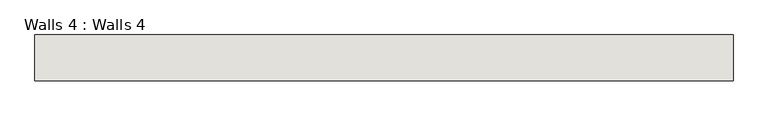
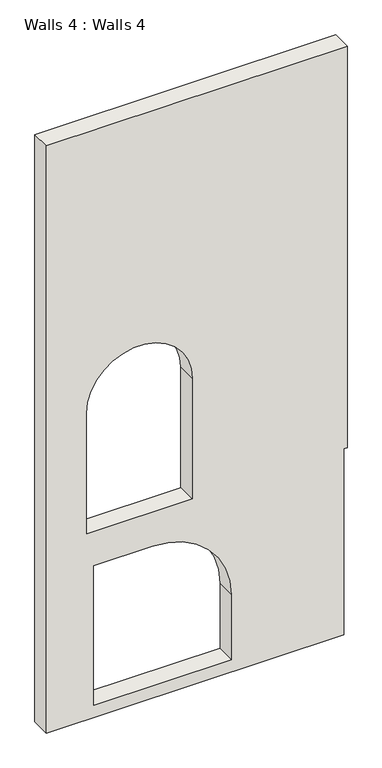
"""IFC4 building model written with IfcOpenShell, lengths in millimetres: wall geometry, Walls 4 : Walls 4."""

from ifc_helpers import new_model, si_unit, point, frame, frame_2d, origin, place, context, project, spatial, polyline, circle_curve, trimmed, segment, composite_curve, outline, extrude, source, transform, mapped, element, save


def walls_4_walls_4_52940900(model_context):
    return source(origin(), model_context, "Body", "SweptSolid", [
        extrude(outline(polyline([(3048.0, 2910.8751902), (3048.0, 7525.9159626), (6096.0, 7525.9159626), (6096.0, 7578.3159626), (12682.2522478, 7578.3159626), (12682.2522478, 2910.8751902), (3048.0, 2910.8751902)]), holes=[composite_curve([segment(trimmed(circle_curve(frame_2d((8077.2, 4355.4054345)), 818.8389056), [point((8077.2, 3536.5665289))], [point((8077.2, 5174.24434))], True, "CARTESIAN"), True, "CONTINUOUS"), segment(polyline([(8077.2, 5174.24434), (6096.0, 5174.24434), (6096.0, 3536.5665289), (8077.2, 3536.5665289)]), True, "CONTINUOUS")], self_intersect=False), composite_curve([segment(polyline([(5533.1852527, 3647.5147473), (5533.1852527, 4564.64434)]), True, "CONTINUOUS"), segment(trimmed(circle_curve(frame_2d((4313.9852527, 4564.64434)), 1219.2), [point((5533.1852527, 4564.64434))], [point((4313.9852527, 5783.84434))], True, "CARTESIAN"), True, "CONTINUOUS"), segment(polyline([(4313.9852527, 5783.84434), (3247.1852527, 5783.84434), (3247.1852527, 3647.5147473), (5533.1852527, 3647.5147473)]), True, "CONTINUOUS")], self_intersect=False)]), frame((0.0, -1198.7851555, 0.0), z_axis=(0.0, 1.0, 0.0), x_axis=(0.0, 0.0, 1.0)), (0.0, 0.0, 1.0), 304.8),
    ])


if __name__ == "__main__":
    model = new_model("IFC4")
    model_context = context("Model", 3, world=origin())
    ifc_project = project(units=[si_unit("LENGTHUNIT", "METRE", prefix="MILLI")], contexts=[model_context])
    site = spatial("IfcSite", under=ifc_project)
    building = spatial("IfcBuilding", under=site)
    placement = place(None, origin())
    walls_4_walls_4_shape = walls_4_walls_4_52940900(model_context)
    element("IfcWall", 1, ObjectType="Walls 4 : Walls 4", at=placement, inside=building, context=model_context, shape_type="MappedRepresentation", body=[
        mapped(walls_4_walls_4_shape, transform((0.0, 0.0, 0.0), x_axis=(1.0, 0.0, 0.0), y_axis=(0.0, 1.0, 0.0), z_axis=(0.0, 0.0, 1.0))),
    ])
    save(model, "model.ifc")

# Revit data of these elements
# Element 1 (IfcWall, "Walls 4 : Walls 4")
#   Materials on its faces: "Default Wall"
# Materials
#   "Default Wall": colour RGB 80 80 80, transparency 0
